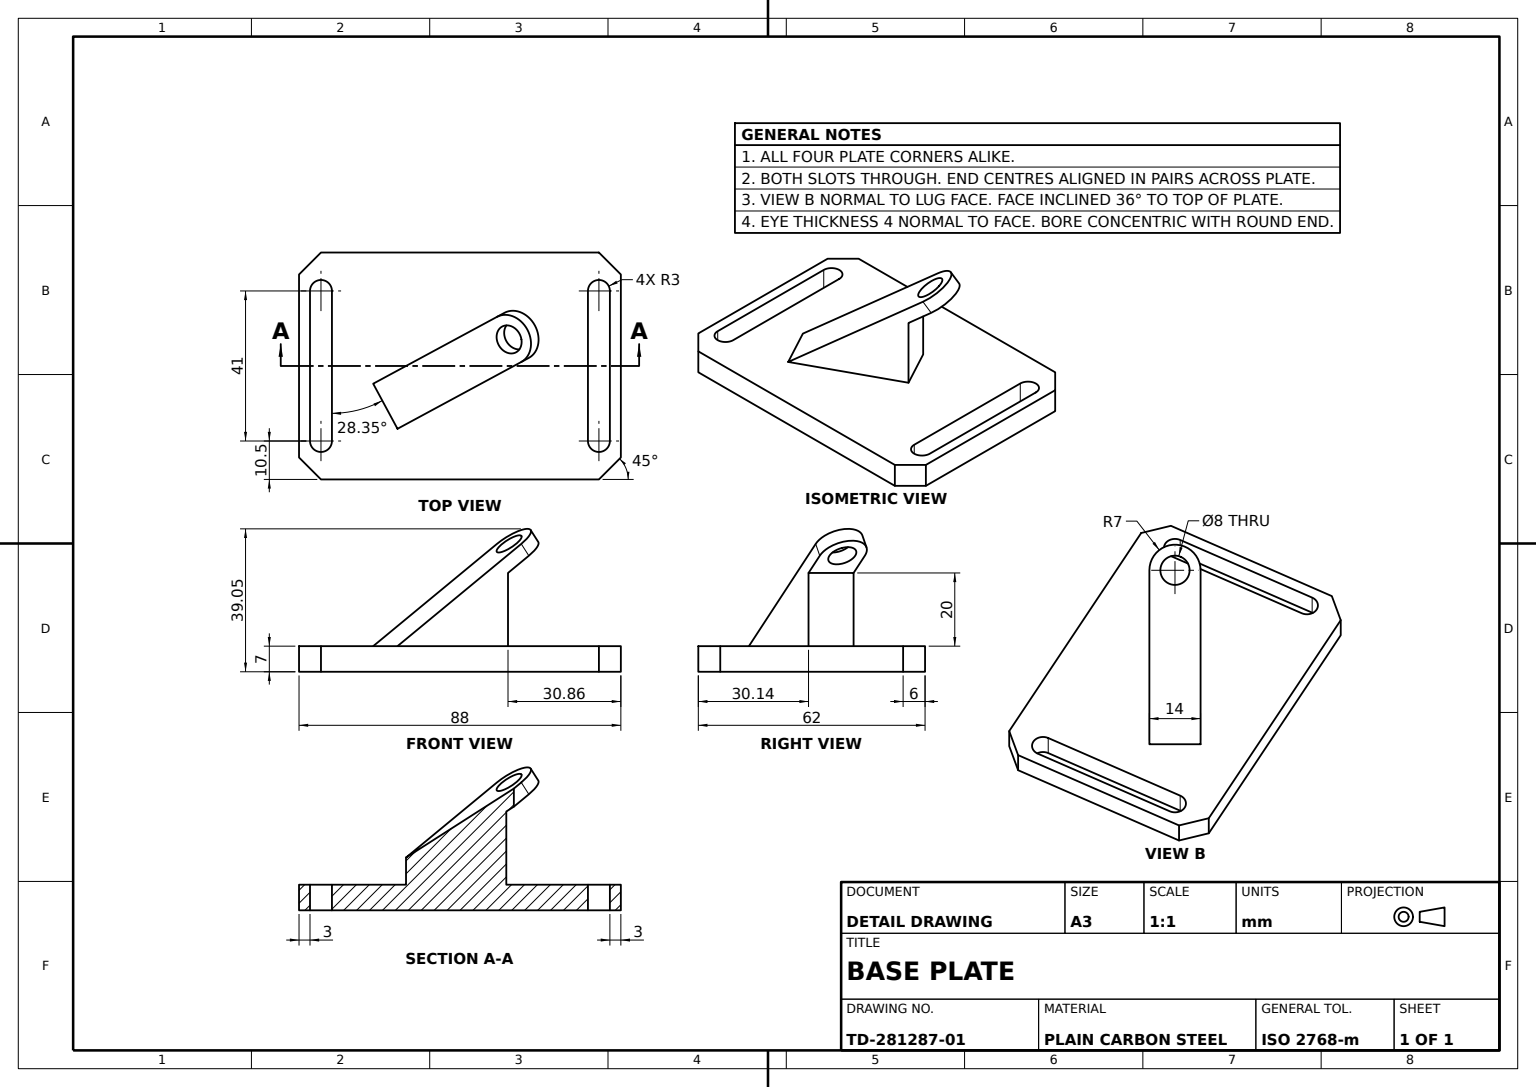
from build123d import *

# Parameters (mm, degrees)
BASE_PLATE_88X62X7_DEPTH = 3.5
LIFTING_LUG_DEPTH        = 7
LUG_EYE_BOSS_SKETCH_R    = 7
LUG_EYE_BOSS_DEPTH       = 4
EYE_HOLE_SKETCH_R        = 4
EYE_HOLE_8_DEPTH         = 4


with BuildPart() as part:
    # Base Plate Sketch → Base Plate 88x62x7 (new, symmetric)
    with BuildSketch(Plane(origin=(0, 0, 0), x_dir=(1, 0, 0), z_dir=(0, 1, 0))):
        Polygon((-44, 25), (-38, 31), (38, 31), (44, 25), (44, -25), (38, -31), (-38, -31), (-44, -25), align=None)
        with BuildLine():
            Line((-41, -20.5), (-41, 20.5))
            ThreePointArc((-41, 20.5), (-38, 23.5), (-35, 20.5))
            Line((-35, 20.5), (-35, -20.5))
            ThreePointArc((-35, -20.5), (-38, -23.5), (-41, -20.5))
        make_face(mode=Mode.SUBTRACT)
        with BuildLine():
            Line((41, -20.5), (41, 20.5))
            ThreePointArc((41, 20.5), (38, 23.5), (35, 20.5))
            Line((35, 20.5), (35, -20.5))
            ThreePointArc((35, -20.5), (38, -23.5), (41, -20.5))
        make_face(mode=Mode.SUBTRACT)
    extrude(amount=BASE_PLATE_88X62X7_DEPTH, both=True)

    # Lug Profile Sketch → Lifting Lug (add, symmetric)
    with BuildSketch(Plane(origin=(0, 0, 0), x_dir=(0.8800989862281835, 0, -0.47479024257046787), z_dir=(0.47479024257046787, 0, 0.8800989862281835))):
        Polygon((-23.176961449, 3.5), (15.276878373, 31.438349996), (17.628019382, 28.202282018), (11.155883427, 23.5), (11.155883427, 3.5), align=None)
    extrude(amount=LIFTING_LUG_DEPTH, both=True)

    # Lug Eye Boss Sketch → Lug Eye Boss (add)
    with BuildSketch(Plane(origin=(-8.512134462, 13.312079847, 4.592072539), x_dir=(0.8557985667033265, 0.4890308937191984, 0.16869380017278038), z_dir=(-0.5173092046624842, 0.8090169943749463, 0.27907470251528765))):
        with Locations((25.657088578, 17.108817488)):
            Circle(LUG_EYE_BOSS_SKETCH_R)
    extrude(amount=-LUG_EYE_BOSS_DEPTH)

    # Eye Hole Sketch → Eye Hole Ø8 (cut)
    with BuildSketch(Plane(origin=(-8.512134462, 13.312079847, 4.592072539), x_dir=(0.8557985667033265, 0.4890308937191984, 0.16869380017278038), z_dir=(-0.5173092046624842, 0.8090169943749463, 0.27907470251528765))):
        with Locations(Location((25.657088578, 17.108817488, 0), (0, 0, 190.117848847))):
            Circle(EYE_HOLE_SKETCH_R)
    extrude(amount=-EYE_HOLE_8_DEPTH, mode=Mode.SUBTRACT)


solid = part.part
